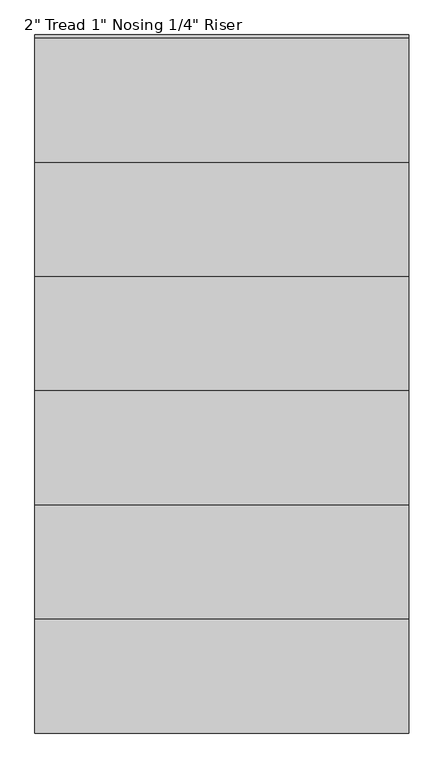
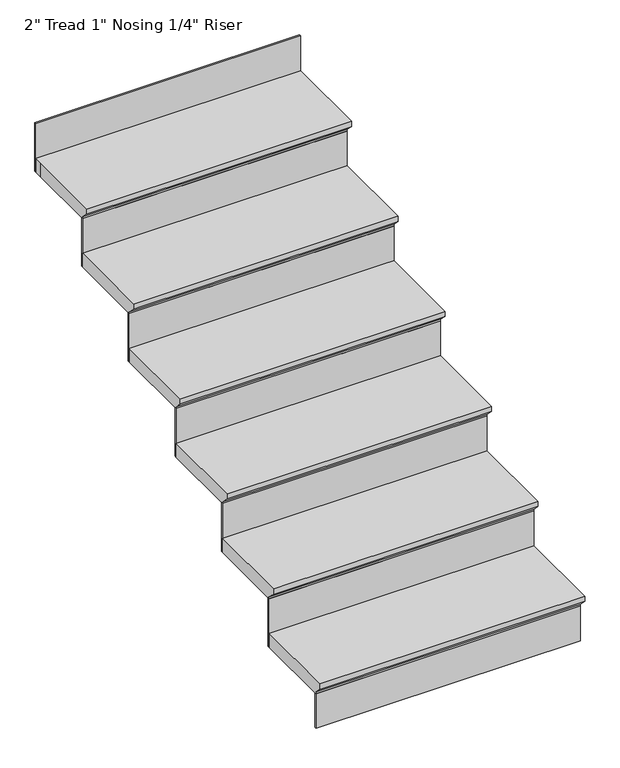
"""IFC4 building model written with IfcOpenShell, lengths in millimetres: stair flight geometry."""

from ifc_helpers import new_model, si_unit, origin, place, context, project, spatial, faceted_brep, source, transform, mapped, element, save


def stair_flight_bb9b06f6(model_context):
    return source(origin(), model_context, "Body", "Brep", [
        faceted_brep([(-12728.1167709, 1039.4362133, 158.75), (-12728.1167709, 1039.4362133, 177.8), (-13642.5167709, 1039.4362133, 177.8), (-13642.5167709, 1039.4362133, 158.75), (-12728.1167709, 1064.8362133, 133.35), (-13642.5167709, 1064.8362133, 133.35), (-12728.1167709, 1344.2362133, 177.8), (-13642.5167709, 1344.2362133, 177.8), (-13642.5167709, 1064.8362133, 127.0), (-13642.5167709, 1344.2362133, 127.0), (-12728.1167709, 1344.2362133, 127.0), (-12728.1167709, 1064.8362133, 127.0)], [[[0, 1, 2, 3]], [[4, 0, 3, 5]], [[2, 1, 6, 7]], [[8, 9, 10, 11]], [[2, 7, 9, 8, 5, 3]], [[8, 11, 4, 5]], [[6, 1, 0, 4, 11, 10]], [[7, 6, 10, 9]]]),
        faceted_brep([(-12728.1167709, 1064.8362133, 127.0), (-12728.1167709, 1064.8362133, 0.0), (-12728.1167709, 1071.1862133, 0.0), (-12728.1167709, 1071.1862133, 127.0), (-13642.5167709, 1064.8362133, 127.0), (-13642.5167709, 1071.1862133, 127.0), (-13642.5167709, 1071.1862133, 0.0), (-13642.5167709, 1064.8362133, 0.0)], [[[0, 1, 2, 3]], [[4, 5, 6, 7]], [[1, 0, 4, 7]], [[2, 1, 7, 6]], [[3, 2, 6, 5]], [[0, 3, 5, 4]]]),
        faceted_brep([(-12728.1167709, 1344.2362133, 304.8), (-12728.1167709, 1344.2362133, 127.0), (-12728.1167709, 1350.5862133, 127.0), (-12728.1167709, 1350.5862133, 304.8), (-13642.5167709, 1344.2362133, 304.8), (-13642.5167709, 1350.5862133, 304.8), (-13642.5167709, 1350.5862133, 127.0), (-13642.5167709, 1344.2362133, 127.0)], [[[0, 1, 2, 3]], [[4, 5, 6, 7]], [[1, 0, 4, 7]], [[2, 1, 7, 6]], [[3, 2, 6, 5]], [[0, 3, 5, 4]]]),
        faceted_brep([(-13642.5167709, 1318.8362133, 355.6), (-12728.1167709, 1318.8362133, 355.6), (-12728.1167709, 1623.6362133, 355.6), (-13642.5167709, 1623.6362133, 355.6), (-13642.5167709, 1344.2362133, 304.8), (-13642.5167709, 1623.6362133, 304.8), (-12728.1167709, 1623.6362133, 304.8), (-12728.1167709, 1344.2362133, 304.8), (-13642.5167709, 1344.2362133, 311.15), (-13642.5167709, 1318.8362133, 336.55), (-12728.1167709, 1344.2362133, 311.15), (-12728.1167709, 1318.8362133, 336.55)], [[[0, 1, 2, 3]], [[4, 5, 6, 7]], [[0, 3, 5, 4, 8, 9]], [[4, 7, 10, 8]], [[2, 1, 11, 10, 7, 6]], [[3, 2, 6, 5]], [[11, 1, 0, 9]], [[10, 11, 9, 8]]]),
        faceted_brep([(-12728.1167709, 1623.6362133, 482.6), (-12728.1167709, 1623.6362133, 304.8), (-12728.1167709, 1629.9862133, 304.8), (-12728.1167709, 1629.9862133, 482.6), (-13642.5167709, 1623.6362133, 482.6), (-13642.5167709, 1629.9862133, 482.6), (-13642.5167709, 1629.9862133, 304.8), (-13642.5167709, 1623.6362133, 304.8)], [[[0, 1, 2, 3]], [[4, 5, 6, 7]], [[1, 0, 4, 7]], [[2, 1, 7, 6]], [[3, 2, 6, 5]], [[0, 3, 5, 4]]]),
        faceted_brep([(-13642.5167709, 1598.2362133, 533.4), (-12728.1167709, 1598.2362133, 533.4), (-12728.1167709, 1903.0362133, 533.4), (-13642.5167709, 1903.0362133, 533.4), (-13642.5167709, 1623.6362133, 482.6), (-13642.5167709, 1903.0362133, 482.6), (-12728.1167709, 1903.0362133, 482.6), (-12728.1167709, 1623.6362133, 482.6), (-13642.5167709, 1623.6362133, 488.95), (-13642.5167709, 1598.2362133, 514.35), (-12728.1167709, 1623.6362133, 488.95), (-12728.1167709, 1598.2362133, 514.35)], [[[0, 1, 2, 3]], [[4, 5, 6, 7]], [[0, 3, 5, 4, 8, 9]], [[4, 7, 10, 8]], [[2, 1, 11, 10, 7, 6]], [[3, 2, 6, 5]], [[11, 1, 0, 9]], [[10, 11, 9, 8]]]),
        faceted_brep([(-12728.1167709, 1903.0362133, 660.4), (-12728.1167709, 1903.0362133, 482.6), (-12728.1167709, 1909.3862133, 482.6), (-12728.1167709, 1909.3862133, 660.4), (-13642.5167709, 1903.0362133, 660.4), (-13642.5167709, 1909.3862133, 660.4), (-13642.5167709, 1909.3862133, 482.6), (-13642.5167709, 1903.0362133, 482.6)], [[[0, 1, 2, 3]], [[4, 5, 6, 7]], [[1, 0, 4, 7]], [[2, 1, 7, 6]], [[3, 2, 6, 5]], [[0, 3, 5, 4]]]),
        faceted_brep([(-13642.5167709, 1877.6362133, 711.2), (-12728.1167709, 1877.6362133, 711.2), (-12728.1167709, 2182.4362133, 711.2), (-13642.5167709, 2182.4362133, 711.2), (-13642.5167709, 1903.0362133, 660.4), (-13642.5167709, 2182.4362133, 660.4), (-12728.1167709, 2182.4362133, 660.4), (-12728.1167709, 1903.0362133, 660.4), (-13642.5167709, 1903.0362133, 666.75), (-13642.5167709, 1877.6362133, 692.15), (-12728.1167709, 1903.0362133, 666.75), (-12728.1167709, 1877.6362133, 692.15)], [[[0, 1, 2, 3]], [[4, 5, 6, 7]], [[0, 3, 5, 4, 8, 9]], [[4, 7, 10, 8]], [[2, 1, 11, 10, 7, 6]], [[3, 2, 6, 5]], [[11, 1, 0, 9]], [[10, 11, 9, 8]]]),
        faceted_brep([(-12728.1167709, 2182.4362133, 838.2), (-12728.1167709, 2182.4362133, 660.4), (-12728.1167709, 2188.7862133, 660.4), (-12728.1167709, 2188.7862133, 838.2), (-13642.5167709, 2182.4362133, 838.2), (-13642.5167709, 2188.7862133, 838.2), (-13642.5167709, 2188.7862133, 660.4), (-13642.5167709, 2182.4362133, 660.4)], [[[0, 1, 2, 3]], [[4, 5, 6, 7]], [[1, 0, 4, 7]], [[2, 1, 7, 6]], [[3, 2, 6, 5]], [[0, 3, 5, 4]]]),
        faceted_brep([(-13642.5167709, 2157.0362133, 889.0), (-12728.1167709, 2157.0362133, 889.0), (-12728.1167709, 2461.8362133, 889.0), (-13642.5167709, 2461.8362133, 889.0), (-13642.5167709, 2182.4362133, 838.2), (-13642.5167709, 2461.8362133, 838.2), (-12728.1167709, 2461.8362133, 838.2), (-12728.1167709, 2182.4362133, 838.2), (-13642.5167709, 2182.4362133, 844.55), (-13642.5167709, 2157.0362133, 869.95), (-12728.1167709, 2182.4362133, 844.55), (-12728.1167709, 2157.0362133, 869.95)], [[[0, 1, 2, 3]], [[4, 5, 6, 7]], [[0, 3, 5, 4, 8, 9]], [[4, 7, 10, 8]], [[2, 1, 11, 10, 7, 6]], [[3, 2, 6, 5]], [[11, 1, 0, 9]], [[10, 11, 9, 8]]]),
        faceted_brep([(-12728.1167709, 2741.2362133, 1193.8), (-12728.1167709, 2741.2362133, 1016.0), (-12728.1167709, 2747.5862133, 1016.0), (-12728.1167709, 2747.5862133, 1193.8), (-13642.5167709, 2741.2362133, 1193.8), (-13642.5167709, 2747.5862133, 1193.8), (-13642.5167709, 2747.5862133, 1016.0), (-13642.5167709, 2741.2362133, 1016.0)], [[[0, 1, 2, 3]], [[4, 5, 6, 7]], [[1, 0, 4, 7]], [[2, 1, 7, 6]], [[3, 2, 6, 5]], [[0, 3, 5, 4]]]),
        faceted_brep([(-12728.1167709, 2461.8362133, 1016.0), (-12728.1167709, 2461.8362133, 838.2), (-12728.1167709, 2468.1862133, 838.2), (-12728.1167709, 2468.1862133, 1016.0), (-13642.5167709, 2461.8362133, 1016.0), (-13642.5167709, 2468.1862133, 1016.0), (-13642.5167709, 2468.1862133, 838.2), (-13642.5167709, 2461.8362133, 838.2)], [[[0, 1, 2, 3]], [[4, 5, 6, 7]], [[1, 0, 4, 7]], [[2, 1, 7, 6]], [[3, 2, 6, 5]], [[0, 3, 5, 4]]]),
        faceted_brep([(-13642.5167709, 2741.2362133, 1066.8), (-13642.5167709, 2715.8362133, 1066.8), (-13642.5167709, 2436.4362133, 1066.8), (-12728.1167709, 2436.4362133, 1066.8), (-12728.1167709, 2715.8362133, 1066.8), (-12728.1167709, 2741.2362133, 1066.8), (-13642.5167709, 2715.8362133, 1016.0), (-13642.5167709, 2741.2362133, 1016.0), (-12728.1167709, 2741.2362133, 1016.0), (-12728.1167709, 2715.8362133, 1016.0), (-12728.1167709, 2461.8362133, 1016.0), (-13642.5167709, 2461.8362133, 1016.0), (-13642.5167709, 2461.8362133, 1022.35), (-13642.5167709, 2436.4362133, 1047.75), (-12728.1167709, 2461.8362133, 1022.35), (-12728.1167709, 2436.4362133, 1047.75)], [[[0, 1, 2, 3, 4, 5]], [[6, 7, 8, 9, 10, 11]], [[1, 0, 7, 6]], [[2, 1, 6, 11, 12, 13]], [[11, 10, 14, 12]], [[4, 3, 15, 14, 10, 9]], [[5, 4, 9, 8]], [[0, 5, 8, 7]], [[15, 3, 2, 13]], [[14, 15, 13, 12]]]),
    ])


if __name__ == "__main__":
    model = new_model("IFC4")
    model_context = context("Model", 3, world=origin())
    ifc_project = project(units=[si_unit("LENGTHUNIT", "METRE", prefix="MILLI")], contexts=[model_context])
    site = spatial("IfcSite", under=ifc_project)
    building = spatial("IfcBuilding", under=site)
    placement = place(None, origin())
    stair_flight_shape = stair_flight_bb9b06f6(model_context)
    element("IfcStairFlight", 1, ObjectType="2\" Tread 1\" Nosing 1/4\" Riser", at=placement, inside=building, context=model_context, shape_type="MappedRepresentation", body=[
        mapped(stair_flight_shape, transform((0.0, 0.0, 0.0), x_axis=(1.0, 0.0, 0.0), y_axis=(0.0, 1.0, 0.0), z_axis=(0.0, 0.0, 1.0))),
    ])
    save(model, "model.ifc")
